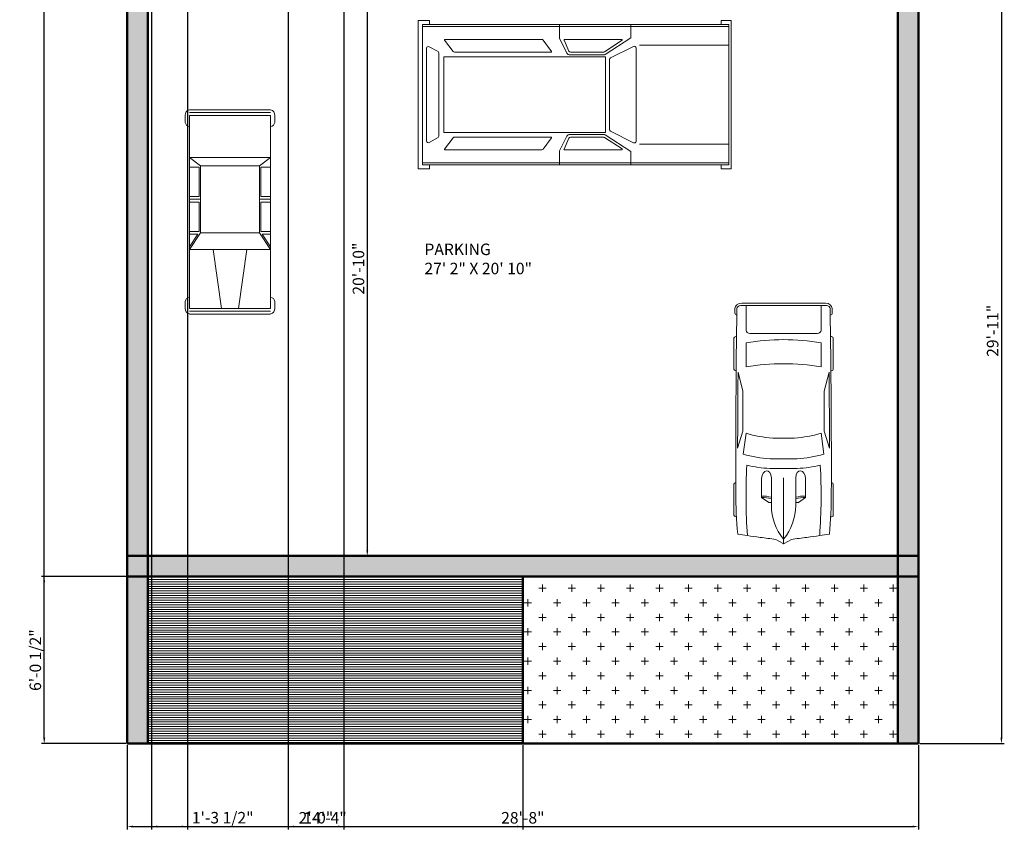
# Model space of a CAD drawing. Units: millimetres. Extents: x 2784 to 3697, y 603 to 1406.
# Tile 1 of 10: x 2784 to 3212, y 603 to 959. Entities that reach past the tile are written whole.
import ezdxf

# ---------------------------------------------------------------- set-up
doc = ezdxf.new("R2010")
doc.units = ezdxf.units.MM
for name, color, linetype, lineweight in [('A-ANNO-DIMS', 140, 'Continuous', 18), ('A-AREA-IDEN', 150, 'Continuous', 25), ('A-EQPM', 9, 'Continuous', 18), ('A-FLOR-PATT', 252, 'Continuous', 13), ('A-WALL', 2, 'Continuous', 50), ('A-WALL-PATT', 8, 'Continuous', 13)]:
    doc.layers.add(name, color=color, linetype=linetype, lineweight=lineweight)
doc.styles.get("Standard").update_dxf_attribs({"font": 'arial.ttf'})
doc.dimstyles.new('ISO-25', dxfattribs={"dimtxt": 5, "dimasz": 2.5, "dimexe": 1.25, "dimexo": 0.625, "dimtad": 1, "dimdec": 0, "dimlunit": 3, "dimtxsty": 'Standard', "dimcen": 2.5, "dimadec": 0, "dimazin": 0, "dimtfac": 1, "dimtdec": 0, "dimtmove": 0, "dimatfit": 3, "dimfxl": 1, "dimarcsym": 0})

# ---------------------------------------------------------------- blocks, each defined once
blk = doc.blocks.new('*U7')
for p, q in [((46.55, 38.89), (22.35, 38.89)), ((136.7, 38.89), (160.9, 38.89)), ((21.1, 37.41), (21.1, 36.83)), ((47.8, 37.39), (47.8, 37.41)), ((70.03, 31.54), (86.41, 29.35)), ((87.99, 31.87), (74.76, 35.92)), ((134.31, 35.6), (119.29, 31.78)), ((135.45, 37.07), (135.45, 37.41)), ((162.15, 37.41), (162.15, 36.77)), ((186.47, -33.5), (186.47, 33.5)), ((188.4, -32.76), (188.4, 32.76)), ((138.42, 29.35), (157.25, 29.35)), ((164.52, 26.39), (164.52, -26.39)), ((186.47, 29.35), (167.01, 29.35)), ((32.27, 11.63), (36.13, 17.17)), ((36.13, 17.17), (50.94, 17.17)), ((29.77, 9.51), (51.68, 9.51)), ((32.12, 9.51), (32.12, 11.15)), ((58.92, -10.77), (58.92, 10.77)), ((66.55, -10.53), (66.55, 10.53)), ((82.74, 8.5), (82.74, -8.5)), ((186.47, -10.53), (186.47, 10.53)), ((3.27, 6.13), (0.1, 0.41)), ((0, 0), (51.68, 0)), ((0.1, -0.41), (3.27, -6.13)), ((29.77, -9.51), (51.68, -9.51)), ((32.12, -9.51), (32.12, -11.15)), ((32.27, -11.63), (36.13, -17.17)), ((36.13, -17.17), (50.94, -17.17)), ((86.41, -29.35), (70.03, -31.54)), ((157.25, -29.35), (138.42, -29.35)), ((167.01, -29.35), (186.47, -29.35)), ((21.1, -37.41), (21.1, -36.83)), ((47.8, -37.39), (47.8, -37.41)), ((87.99, -31.87), (74.76, -35.92)), ((134.31, -35.6), (119.29, -31.78)), ((135.45, -37.07), (135.45, -37.41)), ((162.15, -37.41), (162.15, -36.77)), ((46.55, -38.89), (22.35, -38.89)), ((136.7, -38.89), (160.9, -38.89))]:
    blk.add_line(p, q)
for centre, major_axis, ratio, start_param, end_param in [((22.35, 37.41), (0, -1.48), 0.842304, 3.141593, 4.712389), ((46.55, 37.41), (0, 1.48), 0.842304, -1.570796, 0), ((136.7, 37.41), (0, -1.48), 0.842304, 3.141593, 4.712389), ((160.9, 37.41), (0, 1.48), 0.842304, -1.570796, 0), ((266.03, -27.52), (0, 313.31), 0.842304, 1.367076, 1.39176), ((41.19, -490.86), (0, 528.23), 0.842304, 0.00281, 0.075598), ((64.48, -10555.62), (0, 10593.03), 0.842304, -0.013397, 0.002797), ((135.29, 5.39), (0, 81.77), 0.842304, 1.245306, 1.50788), ((64.48, -10555.62), (0, -10591.55), 0.842304, 3.133765, 3.140441), ((95.79, -3666.35), (0, -3698.24), 0.842304, 3.134049, 3.144098), ((180.63, 35.84), (0, 2.22), 0.842304, -0.013017, 1.249894), ((64.48, -10556.36), (0, 10595.31), 0.842304, -0.013397, -0.013017), ((183.98, 33.5), (0, -2.96), 0.842304, 1.570796, 3.128196), ((183.98, 32.76), (0, -5.25), 0.842304, 1.570796, 3.128196), ((259.18, -27.52), (0, -305.3), 0.842304, 4.528606, 4.561838), ((37.47, -593.96), (0, -623.33), 0.842304, 3.096046, 3.200911), ((134.4, 5.39), (0, -89.78), 0.842304, 4.449482, 4.652344), ((149.6, 2.8), (0, -79.58), 0.842304, 4.372215, 4.640744), ((17.08, 0), (0, 147.02), 0.842304, 4.511394, 4.913384), ((35.91, 0), (0, 147.02), 0.842304, 4.511394, 4.913384), ((167.01, 26.39), (0, 2.96), 0.842304, 0, 1.570796), ((-204.49, 52.4), (0, -250.96), 0.842304, 1.385369, 1.434372), ((13.04, 17.01), (0, 27.42), 0.842304, 4.435146, 4.718221), ((14.2, 17.01), (0, 27.42), 0.842304, 4.435146, 4.718221), ((50.79, 13.34), (6.34, -0.36), 0.603834, -1.395552, 1.581315), ((29.77, -46.66), (0, 56.17), 0.842304, 0, 0.590319), ((32.75, 11.15), (0, 0.74), 0.842304, 0.879714, 1.570796), ((0.62, 0), (0, -0.74), 0.842304, 4.131459, 5.293319), ((-204.49, -52.4), (0, 250.96), 0.842304, -1.434372, -1.385369), ((29.77, 46.66), (0, 56.17), 0.842304, 2.551274, 3.141593), ((32.75, -11.15), (0, -0.74), 0.842304, 4.712389, 5.403472), ((13.04, -17.01), (0, -27.42), 0.842304, 1.564964, 1.848039), ((14.2, -17.01), (0, -27.42), 0.842304, 1.564964, 1.848039), ((134.4, -5.39), (0, -89.78), 0.842304, -1.510751, -1.307889), ((135.29, -5.39), (0, -81.77), 0.842304, -1.50788, -1.245306), ((149.6, -2.8), (0, -79.58), 0.842304, -1.499151, -1.230623), ((259.18, 27.52), (0, 305.3), 0.842304, 1.721348, 1.754579), ((266.03, 27.52), (0, 313.31), 0.842304, 1.749832, 1.774517), ((37.47, 593.96), (0, -623.33), 0.842304, -0.059319, 0.045547), ((167.01, -26.39), (0, -2.96), 0.842304, 4.712389, 6.283185), ((41.19, 490.86), (0, -528.23), 0.842304, -0.075598, -0.00281), ((22.35, -37.41), (0, 1.48), 0.842304, 1.570796, 3.141593), ((64.48, 10555.62), (0, 10593.03), 0.842304, 3.138796, 3.15499), ((46.55, -37.41), (0, -1.48), 0.842304, 0, 1.570796), ((64.48, 10555.62), (0, -10591.55), 0.842304, 0.001152, 0.007828), ((95.79, 3666.35), (0, -3698.24), 0.842304, -0.002505, 0.007544), ((136.7, -37.41), (0, -1.48), 0.842304, -1.570796, 0), ((160.9, -37.41), (0, 1.48), 0.842304, 3.141593, 4.712389), ((180.63, -35.84), (0, -2.22), 0.842304, -1.249894, 0.013017), ((64.48, 10556.36), (0, 10595.31), 0.842304, 3.15461, 3.15499), ((183.98, -33.5), (0, 2.96), 0.842304, 3.15499, 4.712389), ((183.98, -32.76), (0, -5.25), 0.842304, 0.013397, 1.570796)]:
    blk.add_ellipse(centre, major_axis=major_axis, ratio=ratio, start_param=start_param, end_param=end_param)
at = {"extrusion": (0, 0, -1)}
blk.add_ellipse((50.79, -13.34), major_axis=(6.34, 0.36), ratio=0.603834, start_param=-1.395552, end_param=1.581315, dxfattribs=at)
blk = doc.blocks.new('*U8')
for p, q in [((0.1, -0.41), (0.1, 38.35)), ((2.77, -0.41), (2.77, 38.31)), ((5.44, 42.31), (12.12, 42.31)), ((5.44, -0.41), (5.44, 38.24)), ((5.45, 38.31), (16.12, 38.31)), ((16.12, 38.31), (180.34, 38.31)), ((61.52, -0.41), (61.52, 38.31)), ((61.52, 38.31), (77.54, 27.62)), ((64.19, 38.31), (76.2, 30.29)), ((76.2, 30.29), (76.2, 38.31)), ((78.87, 38.31), (78.87, 28.96)), ((106.91, 28.96), (106.91, 38.31)), ((109.58, 27.62), (109.58, 38.31)), ((112.25, 38.31), (112.25, 28.96)), ((140.29, 28.96), (140.29, 38.31)), ((141.62, 27.62), (149.64, 38.31)), ((149.64, -0.41), (149.64, 38.31)), ((189.69, 38.31), (179.01, 38.31)), ((189.69, 42.31), (183.01, 42.31)), ((189.69, -0.41), (189.69, 38.24)), ((192.36, -0.41), (192.36, 38.31)), ((195.03, -0.41), (195.03, 38.35)), ((78.87, 28.96), (106.91, 28.96)), ((112.25, 28.96), (140.29, 28.96)), ((77.54, 27.62), (141.62, 27.62)), ((77.54, -0.41), (77.54, 27.62)), ((141.62, -0.41), (141.62, 27.62)), ((5.44, 7.6), (61.52, 15.61)), ((0.1, -0.42), (0.1, -39.18)), ((2.77, -0.41), (2.77, -39.13)), ((5.44, -0.42), (5.44, -39.07)), ((5.44, -8.42), (61.52, -16.43)), ((61.52, -0.41), (61.52, -39.13)), ((77.54, -0.41), (77.54, -28.45)), ((141.62, -0.41), (141.62, -28.45)), ((149.64, -0.41), (149.64, -39.13)), ((189.69, -0.42), (189.69, -39.07)), ((192.36, -0.41), (192.36, -39.13)), ((195.03, -0.42), (195.03, -39.18)), ((61.52, -39.13), (77.54, -28.45)), ((64.19, -39.13), (76.2, -31.12)), ((76.2, -31.12), (76.2, -39.13)), ((77.54, -28.45), (141.62, -28.45)), ((78.87, -39.13), (78.87, -29.79)), ((78.87, -29.79), (106.91, -29.79)), ((106.91, -29.79), (106.91, -39.13)), ((109.58, -28.45), (109.58, -39.13)), ((112.25, -29.79), (140.29, -29.79)), ((112.25, -39.13), (112.25, -29.79)), ((140.29, -29.79), (140.29, -39.13)), ((141.62, -28.45), (149.64, -39.13)), ((5.44, -43.14), (12.12, -43.14)), ((5.45, -39.13), (16.12, -39.13)), ((16.12, -39.13), (180.34, -39.13)), ((189.69, -39.13), (179.01, -39.13)), ((189.69, -43.14), (183.01, -43.14))]:
    blk.add_line(p, q)
for centre, radius, start, end in [((5.06, 37.26), 5.06, 85.64554, 168.0943), ((11.45, 37.64), 4.72, 8.13011, 81.86996), ((183.68, 37.64), 4.72, 98.13004, 171.8699), ((190.07, 37.26), 5.06, 11.90574, 94.35446), ((5.06, -38.09), 5.06, 191.9057, 274.3545), ((11.45, -38.46), 4.72, 278.13, 351.8699), ((183.68, -38.46), 4.72, 188.1301, 261.87), ((190.07, -38.09), 5.06, 265.6455, 348.0943)]:
    blk.add_arc(centre, radius, start, end)
blk = doc.blocks.new('*U9')
for p, q in [((1.28, 38.87), (175.66, 38.87)), ((1.28, 28.15), (52.13, 28.15)), ((1.28, -28.15), (52.13, -28.15)), ((1.28, -38.87), (175.66, -38.87))]:
    blk.add_line(p, q)
for points in [[(5.57, 40.01), (5.57, 42.18), (0, 42.18), (0, -42.18), (5.57, -42.18), (5.57, -40.01), (1.28, -40.01), (1.28, 40.01)], [(1.28, 40.01), (175.66, 40.01), (175.66, -40.01), (1.28, -40.01)], [(171.74, 40.01), (175.66, 40.01), (175.66, -40.01), (171.74, -40.01), (171.74, -42.18), (178.14, -42.18), (178.14, 42.18), (171.74, 42.18)], [(71.47, 21.48), (163.42, 21.48), (163.42, -21.48), (71.47, -21.48)]]:
    blk.add_lwpolyline(points, close=True)
for points in [[(57.15, 40.01), (57.15, 32.39), (71.72, 22.83, 0.086577), (72.56, 22.68), (91.59, 22.68, 0.227875), (93.54, 23.62), (97.72, 32.11), (97.72, 40.01)], [(57.15, -40.01), (57.15, -32.39), (71.72, -22.83, -0.086577), (72.56, -22.68), (91.59, -22.68, -0.227875), (93.54, -23.62), (97.72, -32.11), (97.72, -40.01)]]:
    blk.add_lwpolyline(points, format="xyb")
for points in [[(62.08, 30.95), (72.14, 24.35, 0.146139), (72.69, 24.18), (91.42, 24.18, 0.29766), (92.33, 24.78), (95.09, 31.05, 0.541236), (94.86, 31.41), (62.21, 31.41, 0.744989)], [(102.19, 24.58), (106.97, 31, -0.236929), (107.78, 31.41), (162.91, 31.41, -0.621576), (163.11, 31), (158.19, 24.58, -0.233368), (157.39, 24.18), (102.39, 24.18, -0.616908)], [(55.49, 27.42), (68.59, 20.89, -0.284287), (69.14, 19.99), (69.14, -19.99, -0.284287), (68.59, -20.89), (55.49, -27.42, -0.557284), (54.05, -26.53), (54.05, 26.53, -0.557284)], [(171.88, 27.31), (166.83, 24.47, 0.271143), (166.32, 23.6), (166.32, -23.6, 0.271143), (166.83, -24.47), (171.88, -27.31, 0.573387), (173.37, -26.44), (173.37, 26.44, 0.573387)], [(62.08, -30.95), (72.14, -24.35, -0.146139), (72.69, -24.18), (91.42, -24.18, -0.29766), (92.33, -24.78), (95.09, -31.05, -0.541236), (94.86, -31.41), (62.21, -31.41, -0.744989)], [(102.19, -24.58), (106.97, -31, 0.236929), (107.78, -31.41), (162.91, -31.41, 0.621576), (163.11, -31), (158.19, -24.58, 0.233368), (157.39, -24.18), (102.39, -24.18, 0.616908)]]:
    blk.add_lwpolyline(points, format="xyb", close=True)
blk = doc.blocks.new('*D34')
at = {"layer": 'A-ANNO-DIMS', "color": 0, "lineweight": -2, "transparency": 16777216}
for p, q in [((2935.27, 972.73), (2935.27, 727.73)), ((2935.34, 975.23), (2936.52, 975.23)), ((2935.34, 725.23), (2936.52, 725.23))]:
    blk.add_line(p, q, dxfattribs=at)
at = {"layer": 'A-ANNO-DIMS', "color": 0, "transparency": 16777216}
for points in [[(2934.85, 972.73), (2935.69, 972.73), (2935.27, 975.23)], [(2934.85, 727.73), (2935.69, 727.73), (2935.27, 725.23)]]:
    blk.add_solid(points, dxfattribs=at)
at = {"layer": 'Defpoints', "color": 0, "transparency": 16777216}
for p in [(2934.71, 975.23), (2934.71, 725.23), (2935.27, 725.23)]:
    blk.add_point(p, dxfattribs=at)
at = {"layer": 'A-ANNO-DIMS', "color": 0, "transparency": 16777216, "insert": (2932.09, 850.23), "char_height": 5, "attachment_point": 5, "rotation": 90}
blk.add_mtext('20\'-10"', dxfattribs=at)
blk = doc.blocks.new('*D83')
at = {"layer": 'A-ANNO-DIMS', "color": 0, "lineweight": -2, "transparency": 16777216}
for p, q in [((2830.91, 642.97), (2830.91, 606.25)), ((3002.91, 642.97), (3002.91, 606.25)), ((2833.41, 607.5), (3000.41, 607.5))]:
    blk.add_line(p, q, dxfattribs=at)
at = {"layer": 'A-ANNO-DIMS', "color": 0, "transparency": 16777216}
for points in [[(2833.41, 607.91), (2833.41, 607.08), (2830.91, 607.5)], [(3000.41, 607.91), (3000.41, 607.08), (3002.91, 607.5)]]:
    blk.add_solid(points, dxfattribs=at)
at = {"layer": 'Defpoints', "color": 0, "transparency": 16777216}
for p in [(2830.91, 643.6), (3002.91, 643.6), (3002.91, 607.5)]:
    blk.add_point(p, dxfattribs=at)
at = {"layer": 'A-ANNO-DIMS', "color": 0, "transparency": 16777216, "insert": (2916.91, 610.63), "char_height": 5, "attachment_point": 5}
blk.add_mtext('14\'-4"', dxfattribs=at)
blk = doc.blocks.new('*D84')
at = {"layer": 'A-ANNO-DIMS', "color": 0, "lineweight": -2, "transparency": 16777216}
for p, q in [((2830.91, 642.97), (2830.91, 606.25)), ((3174.91, 642.97), (3174.91, 606.25)), ((2833.41, 607.5), (3172.41, 607.5))]:
    blk.add_line(p, q, dxfattribs=at)
at = {"layer": 'A-ANNO-DIMS', "color": 0, "transparency": 16777216}
for points in [[(2833.41, 607.91), (2833.41, 607.08), (2830.91, 607.5)], [(3172.41, 607.91), (3172.41, 607.08), (3174.91, 607.5)]]:
    blk.add_solid(points, dxfattribs=at)
at = {"layer": 'Defpoints', "color": 0, "transparency": 16777216}
for p in [(2830.91, 643.6), (3174.91, 643.6), (3174.91, 607.5)]:
    blk.add_point(p, dxfattribs=at)
at = {"layer": 'A-ANNO-DIMS', "color": 0, "transparency": 16777216, "insert": (3002.91, 610.67), "char_height": 5, "attachment_point": 5}
blk.add_mtext('28\'-8"', dxfattribs=at)
blk = doc.blocks.new('*D85')
at = {"layer": 'A-ANNO-DIMS', "color": 0, "lineweight": -2, "transparency": 16777216}
for p, q in [((2830.28, 716.23), (2793.56, 716.23)), ((2794.81, 646.1), (2794.81, 713.73)), ((2830.28, 643.6), (2793.56, 643.6))]:
    blk.add_line(p, q, dxfattribs=at)
at = {"layer": 'A-ANNO-DIMS', "color": 0, "transparency": 16777216}
for points in [[(2794.39, 713.73), (2795.22, 713.73), (2794.81, 716.23)], [(2794.39, 646.1), (2795.22, 646.1), (2794.81, 643.6)]]:
    blk.add_solid(points, dxfattribs=at)
at = {"layer": 'Defpoints', "color": 0, "transparency": 16777216}
for p in [(2794.81, 716.23), (2830.91, 716.23), (2830.91, 643.6)]:
    blk.add_point(p, dxfattribs=at)
at = {"layer": 'A-ANNO-DIMS', "color": 0, "transparency": 16777216, "insert": (2791.6, 679.91), "char_height": 5, "attachment_point": 5, "rotation": 90}
blk.add_mtext('6\'-0 1/2"', dxfattribs=at)
blk = doc.blocks.new('*D90')
at = {"layer": 'A-ANNO-DIMS', "color": 0, "lineweight": -2, "transparency": 16777216}
for p, q in [((2830.28, 1356.23), (2793.56, 1356.23)), ((2794.81, 646.1), (2794.81, 1353.73)), ((2830.28, 643.6), (2793.56, 643.6))]:
    blk.add_line(p, q, dxfattribs=at)
at = {"layer": 'A-ANNO-DIMS', "color": 0, "transparency": 16777216}
for points in [[(2794.39, 1353.73), (2795.22, 1353.73), (2794.81, 1356.23)], [(2794.39, 646.1), (2795.22, 646.1), (2794.81, 643.6)]]:
    blk.add_solid(points, dxfattribs=at)
at = {"layer": 'Defpoints', "color": 0, "transparency": 16777216}
for p in [(2794.81, 1356.23), (2830.91, 1356.23), (2830.91, 643.6)]:
    blk.add_point(p, dxfattribs=at)
at = {"layer": 'A-ANNO-DIMS', "color": 0, "transparency": 16777216, "insert": (2791.6, 999.91), "char_height": 5, "attachment_point": 5, "rotation": 90}
blk.add_mtext('59\'-4 1/2"', dxfattribs=at)
blk = doc.blocks.new('*D99')
at = {"layer": 'A-ANNO-DIMS', "color": 0, "lineweight": -2, "transparency": 16777216}
for p, q in [((3175.53, 1002.74), (3212.26, 1002.74)), ((3211.01, 1000.24), (3211.01, 646.1)), ((3175.53, 643.6), (3212.26, 643.6))]:
    blk.add_line(p, q, dxfattribs=at)
at = {"layer": 'A-ANNO-DIMS', "color": 0, "transparency": 16777216}
for points in [[(3210.59, 1000.24), (3211.42, 1000.24), (3211.01, 1002.74)], [(3210.59, 646.1), (3211.42, 646.1), (3211.01, 643.6)]]:
    blk.add_solid(points, dxfattribs=at)
at = {"layer": 'Defpoints', "color": 0, "transparency": 16777216}
for p in [(3174.91, 1002.74), (3174.91, 643.6), (3211.01, 643.6)]:
    blk.add_point(p, dxfattribs=at)
at = {"layer": 'A-ANNO-DIMS', "color": 0, "transparency": 16777216, "insert": (3207.83, 823.17), "char_height": 5, "attachment_point": 5, "rotation": 90}
blk.add_mtext('29\'-11"', dxfattribs=at)
blk = doc.blocks.new('*D102')
at = {"layer": 'A-ANNO-DIMS', "color": 0, "lineweight": -2, "transparency": 16777216}
for p, q in [((2841.43, 974.52), (2841.43, 606.25)), ((2857.05, 974.52), (2857.05, 606.25)), ((2843.93, 607.5), (2854.55, 607.5)), ((2857.05, 607.5), (2885.27, 607.5))]:
    blk.add_line(p, q, dxfattribs=at)
at = {"layer": 'A-ANNO-DIMS', "color": 0, "transparency": 16777216}
for points in [[(2843.93, 607.91), (2843.93, 607.08), (2841.43, 607.5)], [(2854.55, 607.91), (2854.55, 607.08), (2857.05, 607.5)]]:
    blk.add_solid(points, dxfattribs=at)
at = {"layer": 'Defpoints', "color": 0, "transparency": 16777216}
for p in [(2841.43, 975.14), (2857.05, 975.14), (2857.05, 607.5)]:
    blk.add_point(p, dxfattribs=at)
at = {"layer": 'A-ANNO-DIMS', "color": 0, "transparency": 16777216, "insert": (2872.41, 610.71), "char_height": 5, "attachment_point": 5}
blk.add_mtext('1\'-3 1/2"', dxfattribs=at)
blk = doc.blocks.new('*D103')
at = {"layer": 'A-ANNO-DIMS', "color": 0, "lineweight": -2, "transparency": 16777216}
for p, q in [((2900.85, 974.61), (2900.85, 606.25)), ((2925.01, 974.61), (2925.01, 606.25)), ((2903.35, 607.5), (2922.51, 607.5))]:
    blk.add_line(p, q, dxfattribs=at)
at = {"layer": 'A-ANNO-DIMS', "color": 0, "transparency": 16777216}
for points in [[(2903.35, 607.91), (2903.35, 607.08), (2900.85, 607.5)], [(2922.51, 607.91), (2922.51, 607.08), (2925.01, 607.5)]]:
    blk.add_solid(points, dxfattribs=at)
at = {"layer": 'Defpoints', "color": 0, "transparency": 16777216}
for p in [(2900.85, 975.23), (2925.01, 975.23), (2925.01, 607.5)]:
    blk.add_point(p, dxfattribs=at)
at = {"layer": 'A-ANNO-DIMS', "color": 0, "transparency": 16777216, "insert": (2912.93, 610.67), "char_height": 5, "attachment_point": 5}
blk.add_mtext('2\'-0"', dxfattribs=at)

msp = doc.modelspace()

# ---------------------------------------------------------------- hatches: boundary and pattern name
at = {"layer": 'A-FLOR-PATT'}
h = msp.add_hatch(dxfattribs=at)
h.set_pattern_fill('ANSI31', color=256, scale=0.314961, angle=-45, style=0)
h.paths.add_polyline_path([(2839.91, 643.6), (3002.91, 643.6), (3002.91, 715.6), (2839.91, 715.6)])
h = msp.add_hatch(dxfattribs=at)
h.set_pattern_fill('CROSS', color=256)
h.paths.add_polyline_path([(3165.91, 716.23), (3002.91, 716.23), (3002.91, 643.6), (3165.91, 643.6)])
at = {"layer": 'A-WALL-PATT'}
h = msp.add_hatch(color=256, dxfattribs=at)
h.dxf.hatch_style = 1
h.paths.add_polyline_path([(2869.53, 1356.23), (2839.91, 1356.23), (2839.91, 1347.23), (2869.53, 1347.23)])
h.paths.add_polyline_path([(2839.91, 1356.23), (2830.91, 1356.23), (2830.91, 1347.23), (2839.91, 1347.23)])
h.paths.add_polyline_path([(2839.91, 1347.23), (2830.91, 1347.23), (2830.91, 1314.23), (2839.91, 1314.23)])
h.paths.add_polyline_path([(2839.91, 1268.19), (2830.91, 1268.19), (2830.91, 1222.23), (2839.91, 1222.23)])
h.paths.add_polyline_path([(2839.91, 1222.23), (2830.91, 1222.23), (2830.91, 1213.23), (2839.91, 1213.23)])
h.paths.add_polyline_path([(2962.91, 1222.23), (2839.91, 1222.23), (2839.91, 1213.23), (2962.91, 1213.23)])
h.paths.add_polyline_path([(2971.91, 1222.23), (2962.91, 1222.23), (2962.91, 1213.23), (2971.91, 1213.23)])
h.paths.add_polyline_path([(2971.91, 1263.23), (2962.91, 1263.23), (2962.91, 1254.23), (2971.91, 1254.23)])
h.paths.add_polyline_path([(2971.91, 1347.23), (2962.91, 1347.23), (2962.91, 1263.23), (2971.91, 1263.23)])
h.paths.add_polyline_path([(2971.91, 1356.23), (2962.91, 1356.23), (2962.91, 1347.23), (2971.91, 1347.23)])
h.paths.add_polyline_path([(2962.91, 1356.23), (2913.7, 1356.23), (2913.7, 1347.23), (2962.91, 1347.23)])
h.paths.add_polyline_path([(2982.62, 1356.23), (2971.91, 1356.23), (2971.91, 1347.23), (2982.62, 1347.23)])
h.paths.add_polyline_path([(3019.91, 1356.23), (3004.44, 1356.23), (3004.44, 1347.23), (3019.91, 1347.23)])
h.paths.add_polyline_path([(3028.91, 1356.23), (3019.91, 1356.23), (3019.91, 1347.23), (3028.91, 1347.23)])
h.paths.add_polyline_path([(3028.91, 1347.23), (3019.91, 1347.23), (3019.91, 1287.35, -0.06506), (3026.12, 1288.16), (3028.91, 1288.16)])
h.paths.add_polyline_path([(3019.91, 1263.23), (2971.91, 1263.23), (2971.91, 1254.23), (3019.91, 1254.23)])
h.paths.add_polyline_path([(3028.91, 1263.23), (3019.91, 1263.23), (3019.91, 1254.23), (3028.91, 1254.23)])
h.paths.add_polyline_path([(3028.91, 1254.23), (3019.91, 1254.23), (3019.91, 1222.23), (3028.91, 1222.23)])
h.paths.add_polyline_path([(3028.91, 1222.23), (3019.91, 1222.23), (3019.91, 1213.23), (3028.91, 1213.23)])
h.paths.add_polyline_path([(3165.91, 1222.23), (3060.65, 1222.23, -0.056956), (3061.45, 1215.23), (3061.45, 1213.23), (3165.91, 1213.23)])
h.paths.add_polyline_path([(3080.34, 1356.23), (3028.91, 1356.23), (3028.91, 1347.23), (3080.34, 1347.23)])
h.paths.add_polyline_path([(3174.91, 1347.23), (3165.91, 1347.23), (3165.91, 1311.28), (3174.91, 1311.28)])
h.paths.add_polyline_path([(3174.91, 1356.23), (3165.91, 1356.23), (3165.91, 1347.23), (3174.91, 1347.23)])
h.paths.add_polyline_path([(3165.91, 1356.23), (3123.1, 1356.23), (3123.1, 1347.23), (3165.91, 1347.23)])
h.paths.add_polyline_path([(3174.91, 1266.65), (3165.91, 1266.65), (3165.91, 1222.23), (3174.91, 1222.23)])
h.paths.add_polyline_path([(3174.91, 1222.23), (3165.91, 1222.23), (3165.91, 1213.23), (3174.91, 1213.23)])
h.paths.add_polyline_path([(3174.91, 1213.23), (3165.91, 1213.23), (3165.91, 1194.83), (3174.91, 1194.83)])
h.paths.add_polyline_path([(3105.91, 1182.92, -0.096276), (3096.91, 1180.92), (3096.91, 1148.23), (3105.91, 1148.23)])
h.paths.add_polyline_path([(3105.91, 1213.23), (3096.91, 1213.23), (3096.91, 1205.07), (3105.91, 1205.07)])
h.paths.add_polyline_path([(2971.91, 1213.23), (2962.91, 1213.23), (2962.91, 1161.09), (2971.91, 1161.09)])
h.paths.add_polyline_path([(2839.91, 1213.23), (2830.91, 1213.23), (2830.91, 1157.46), (2839.91, 1157.46)])
h.paths.add_polyline_path([(2839.91, 1108.88), (2830.91, 1108.88), (2830.91, 1042.23), (2839.91, 1042.23)])
h.paths.add_polyline_path([(2839.91, 1042.23), (2830.91, 1042.23), (2830.91, 1033.23), (2839.91, 1033.23)])
h.paths.add_polyline_path([(2881.91, 1042.23), (2839.91, 1042.23), (2839.91, 1033.23), (2881.91, 1033.23)])
h.paths.add_polyline_path([(2996.91, 1042.23), (2890.91, 1042.23), (2890.91, 1033.23), (2996.91, 1033.23)])
h.paths.add_polyline_path([(2890.91, 1042.23), (2881.91, 1042.23), (2881.91, 1033.23), (2890.91, 1033.23)])
h.paths.add_polyline_path([(2890.91, 1033.23), (2881.91, 1033.23), (2881.91, 984.23), (2890.91, 984.23)])
h.paths.add_polyline_path([(2839.91, 1033.23), (2830.91, 1033.23), (2830.91, 984.23), (2839.91, 984.23)])
h.paths.add_polyline_path([(2839.91, 984.23), (2830.91, 984.23), (2830.91, 975.23), (2839.91, 975.23)])
h.paths.add_polyline_path([(2881.91, 984.23), (2854.14, 984.23, -0.154991), (2857.05, 975.23), (2881.91, 975.23)])
h.paths.add_polyline_path([(2890.91, 984.23), (2881.91, 984.23), (2881.91, 975.23), (2890.91, 975.23)])
h.paths.add_polyline_path([(2900.85, 984.23), (2890.91, 984.23), (2890.91, 975.23), (2900.85, 975.23), (2900.85, 975.78)])
h.paths.add_polyline_path([(2996.91, 984.23), (2923.49, 984.23, -0.089525), (2925.01, 975.78), (2925.01, 975.23), (2996.91, 975.23)])
h.paths.add_polyline_path([(3165.91, 984.23), (3005.91, 984.23), (3005.91, 975.23), (3165.91, 975.23)])
h.paths.add_polyline_path([(3005.91, 1033.23), (2996.91, 1033.23), (2996.91, 984.23), (3005.91, 984.23)])
h.paths.add_polyline_path([(3005.91, 984.23), (2996.91, 984.23), (2996.91, 975.23), (3005.91, 975.23)])
h.paths.add_polyline_path([(3005.91, 1042.23), (2996.91, 1042.23), (2996.91, 1033.23), (3005.91, 1033.23)])
h.paths.add_polyline_path([(3096.91, 1079.23), (2971.91, 1079.23), (2971.91, 1070.23), (3096.91, 1070.23)])
h.paths.add_polyline_path([(2971.91, 1079.23), (2962.91, 1079.23), (2962.91, 1070.23), (2971.91, 1070.23)])
h.paths.add_polyline_path([(2971.91, 1070.23), (2962.91, 1070.23), (2962.91, 1060.28, -0.115005), (2971.91, 1066.55)])
h.paths.add_polyline_path([(2971.91, 1105.54), (2962.91, 1105.54), (2962.91, 1079.23), (2971.91, 1079.23)])
h.paths.add_polyline_path([(3165.91, 1079.23), (3105.91, 1079.23), (3105.91, 1070.23), (3165.91, 1070.23)])
h.paths.add_polyline_path([(3105.91, 1079.23), (3096.91, 1079.23), (3096.91, 1070.23), (3105.91, 1070.23)])
h.paths.add_polyline_path([(3105.91, 1148.23), (3096.91, 1148.23), (3096.91, 1139.23), (3105.91, 1139.23)])
h.paths.add_polyline_path([(3105.91, 1139.23), (3096.91, 1139.23), (3096.91, 1104.7), (3098.08, 1104.75, -0.08216), (3105.91, 1103.81)])
h.paths.add_polyline_path([(3165.91, 1148.23), (3105.91, 1148.23), (3105.91, 1139.23), (3165.91, 1139.23)])
h.paths.add_polyline_path([(3174.91, 1148.23), (3165.91, 1148.23), (3165.91, 1139.23), (3174.91, 1139.23)])
h.paths.add_polyline_path([(3174.91, 1139.23), (3165.91, 1139.23), (3165.91, 1123.86), (3174.91, 1123.86)])
h.paths.add_polyline_path([(3174.91, 1097.37), (3165.91, 1097.37), (3165.91, 1079.23), (3174.91, 1079.23)])
h.paths.add_polyline_path([(3174.91, 1079.23), (3165.91, 1079.23), (3165.91, 1070.23), (3174.91, 1070.23)])
h.paths.add_polyline_path([(3174.91, 1070.23), (3165.91, 1070.23), (3165.91, 1048.77), (3174.91, 1048.77)])
h.paths.add_polyline_path([(3174.91, 1002.74), (3165.91, 1002.74), (3165.91, 984.23), (3174.91, 984.23)])
h.paths.add_polyline_path([(3174.91, 984.23), (3165.91, 984.23), (3165.91, 975.23), (3174.91, 975.23)])
h.paths.add_polyline_path([(3174.91, 975.23), (3165.91, 975.23), (3165.91, 725.23), (3174.91, 725.23)])
h.paths.add_polyline_path([(2839.91, 975.23), (2830.91, 975.23), (2830.91, 725.23), (2839.91, 725.23)])
h.paths.add_polyline_path([(3165.91, 725.23), (2839.91, 725.23), (2839.91, 716.23), (3165.91, 716.23)])
h.paths.add_polyline_path([(3174.91, 725.23), (3165.91, 725.23), (3165.91, 716.23), (3174.91, 716.23)])
h.paths.add_polyline_path([(2839.91, 725.23), (2830.91, 725.23), (2830.91, 716.23), (2839.91, 716.23)])
h = msp.add_hatch(color=256, dxfattribs=at)
h.dxf.hatch_style = 1
h.paths.add_polyline_path([(2839.91, 716.23), (2830.91, 716.23), (2830.91, 643.6), (2839.91, 643.6)])
h = msp.add_hatch(color=256, dxfattribs=at)
h.dxf.hatch_style = 1
h.paths.add_polyline_path([(3174.91, 716.23), (3165.91, 716.23), (3165.91, 643.6), (3174.91, 643.6)])

# ---------------------------------------------------------------- linework, layer by layer
at = {"layer": 'A-WALL'}
for p, q in [((2830.91, 1356.23), (2830.91, 716.23)), ((2839.91, 1356.23), (2839.91, 643.6)), ((3165.91, 1213.23), (3165.91, 643.6)), ((3174.91, 1213.23), (3174.91, 643.6)), ((2830.91, 725.23), (3174.91, 725.23)), ((2830.91, 716.23), (3174.91, 716.23)), ((2830.91, 716.23), (2830.91, 643.6)), ((2830.91, 643.6), (3174.91, 643.6))]:
    msp.add_line(p, q, dxfattribs=at)
msp.add_lwpolyline([(2839.91, 716.23), (3002.91, 716.23), (3002.91, 643.6), (2839.91, 643.6)], close=True, dxfattribs=at)

# ---------------------------------------------------------------- block references
at = {"layer": 'A-EQPM'}
for name, p, xscale, yscale, zscale, rotation in [('*U9', (3093.46, 925.93), 0.7638636157426095, 0.7638636157426095, 0.7638636157426095, 180), ('*U8', (2875.4, 830.44), 0.4557687717440757, 0.4557687717440757, 0.4557687717440757, 90), ('*U7', (3116.27, 730.56), 0.5557068697343422, 0.5557068697343422, 0.5557068697343422, 90)]:
    msp.add_blockref(name, p, dxfattribs=dict(at, xscale=xscale, yscale=yscale, zscale=zscale, rotation=rotation))

# ---------------------------------------------------------------- texts
at = {"layer": 'A-AREA-IDEN', "insert": (2960.12, 861.11), "char_height": 5, "attachment_point": 1}
msp.add_mtext_dynamic_manual_height_columns('PARKING \\P27\' 2" X 20\' 10"', width=81.4347, gutter_width=12.5, heights=[0], dxfattribs=at)

# ---------------------------------------------------------------- dimensions: what is measured, and where the dimension line sits
at = {"layer": 'A-ANNO-DIMS'}
for base, p1, p2, override, picture, middle in [((2794.81, 1356.23), (2830.91, 643.6), (2830.91, 1356.23), {"dimdec": 1, "dimlfac": 1, "dimrnd": 0, "dimzin": 1, "dimdsep": 46, "dimlunit": 4, "dimfrac": 2}, '*D90', (2791.6, 999.91)), ((3211.01, 643.6), (3174.91, 1002.74), (3174.91, 643.6), {"dimdec": 1, "dimlfac": 1, "dimrnd": 0, "dimzin": 1, "dimdsep": 46, "dimlunit": 4, "dimfrac": 2}, '*D99', (3207.83, 823.17)), ((2935.27, 725.23), (2934.71, 975.23), (2934.71, 725.23), {"dimclrd": 0, "dimclre": 0, "dimclrt": 0}, '*D34', (2932.09, 850.23)), ((2794.81, 716.23), (2830.91, 643.6), (2830.91, 716.23), {"dimdec": 1, "dimlfac": 1, "dimrnd": 0, "dimzin": 1, "dimdsep": 46, "dimlunit": 4, "dimfrac": 2}, '*D85', (2791.6, 679.91))]:
    dim = msp.add_linear_dim(base=base, p1=p1, p2=p2, angle=90, dimstyle='ISO-25', override=override, dxfattribs=at)
    dim.commit()
    dim.dimension.update_dxf_attribs({"geometry": picture, "text_midpoint": middle})
for base, p1, p2, picture, middle in [((2857.05, 607.5), (2841.43, 975.14), (2857.05, 975.14), '*D102', (2872.41, 610.71)), ((2925.01, 607.5), (2900.85, 975.23), (2925.01, 975.23), '*D103', (2912.93, 610.67)), ((3002.91, 607.5), (2830.91, 643.6), (3002.91, 643.6), '*D83', (2916.91, 610.63)), ((3174.91, 607.5), (2830.91, 643.6), (3174.91, 643.6), '*D84', (3002.91, 610.67))]:
    dim = msp.add_linear_dim(base=base, p1=p1, p2=p2, dimstyle='ISO-25', override={"dimdec": 1, "dimlfac": 1, "dimrnd": 0, "dimzin": 1, "dimdsep": 46, "dimlunit": 4, "dimfrac": 2}, dxfattribs=at)
    dim.commit()
    dim.dimension.update_dxf_attribs({"geometry": picture, "text_midpoint": middle})

doc.saveas('drawing.dxf')
